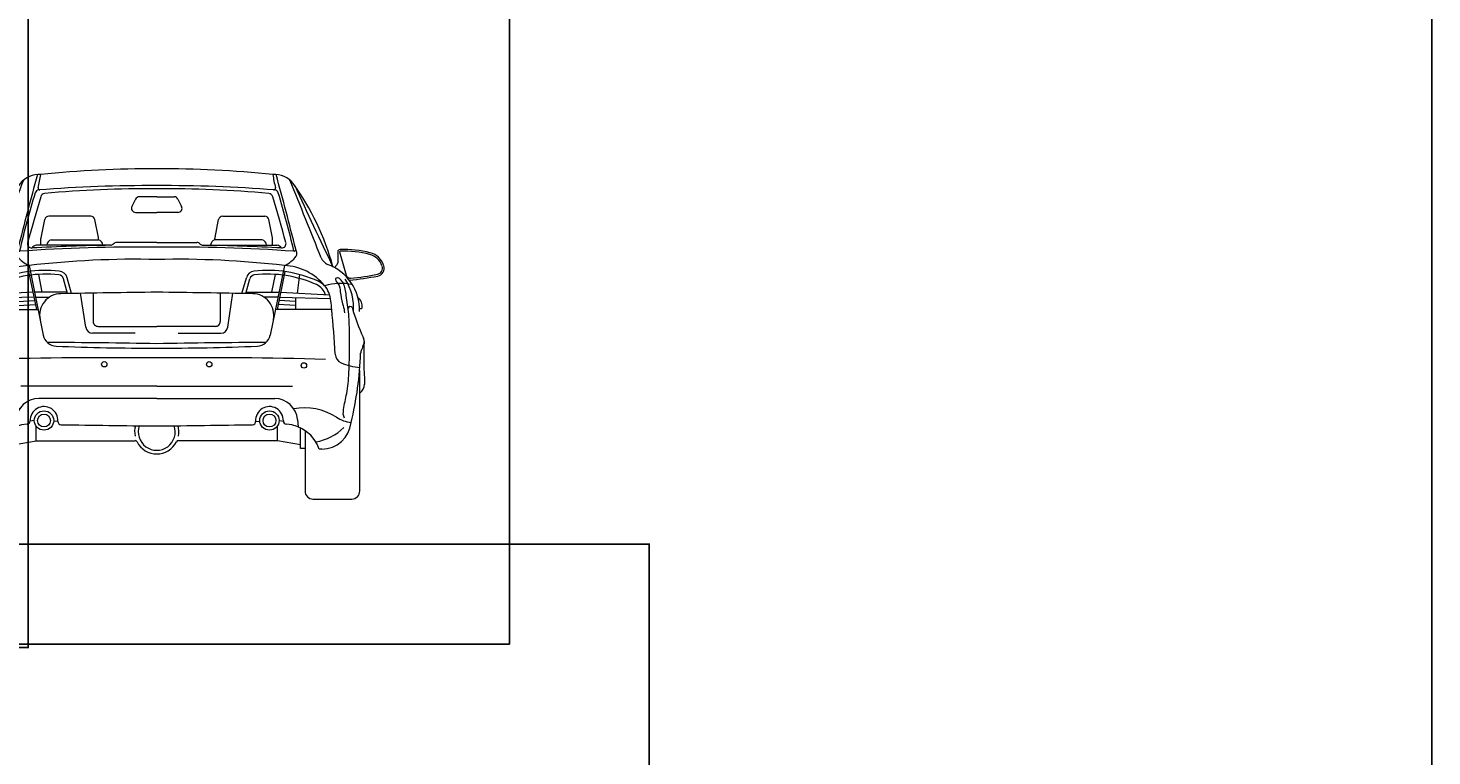
# Model space of a CAD drawing. Units: inches. Extents: x 1770 to 2988, y 1161 to 3221.
# Tile 37 of 44: x 2655 to 2988, y 2520 to 2693. Entities that reach past the tile are written whole.
import ezdxf

# ---------------------------------------------------------------- set-up
doc = ezdxf.new("R2010")
doc.units = ezdxf.units.IN
for name, color, linetype, lineweight in [('A-ANNO-DIMS', 2, 'Continuous', 18), ('A-ANNO-TTLB', 7, 'Continuous', 25), ('AUDI', 8, 'Continuous', 13)]:
    doc.layers.add(name, color=color, linetype=linetype, lineweight=lineweight)
doc.styles.get("Standard").update_dxf_attribs({"font": 'arial.ttf'})
doc.dimstyles.get("Standard").update_dxf_attribs({"dimtxt": 0.18, "dimasz": 0.18, "dimexe": 0.18, "dimexo": 0.0625, "dimgap": 0.09, "dimtad": 0, "dimtih": 1, "dimtoh": 1, "dimdec": 4, "dimzin": 0, "dimdsep": 46, "dimtxsty": 'Standard', "dimcen": 0.09, "dimadec": 0, "dimazin": 0, "dimtfac": 1, "dimtdec": 4, "dimtofl": 0, "dimtmove": 0, "dimatfit": 3, "dimfxl": 1, "dimtolj": 1, "dimtzin": 0, "dimarcsym": 0})

# ---------------------------------------------------------------- blocks, each defined once
blk = doc.blocks.new('CAR-SEDAN-REAR')
for p, q in [((48.82, 70.96), (47.96, 69.22)), ((53.84, 71.5), (49.7, 71.5)), ((53.84, 71.5), (57.98, 71.5)), ((58.85, 70.96), (59.72, 69.22)), ((38.23, 66.92), (28.28, 66.92)), ((48.83, 67.81), (53.84, 67.81)), ((58.85, 67.81), (53.84, 67.81)), ((69.45, 66.92), (79.4, 66.92)), ((26.45, 61.8), (27.32, 66.14)), ((40.05, 61.84), (39.18, 66.14)), ((67.63, 61.84), (68.49, 66.14)), ((81.23, 61.8), (80.35, 66.14)), ((42.86, 60.02), (25.37, 60.02)), ((26.43, 60.02), (26.43, 61.6)), ((28.84, 61.32), (40.07, 61.32)), ((40.07, 61.32), (40.07, 61.65)), ((53.84, 60.68), (44.34, 60.68)), ((53.84, 60.68), (63.33, 60.68)), ((64.82, 60.02), (82.31, 60.02)), ((67.61, 61.32), (67.61, 61.65)), ((78.83, 61.32), (67.61, 61.32)), ((81.25, 60.02), (81.25, 61.6)), ((10.57, 58.46), (8.97, 52.97)), ((10.98, 58.46), (10.98, 55.88)), ((96.69, 58.46), (96.69, 55.88)), ((97.11, 58.46), (98.7, 52.97)), ((11.13, 55.5), (11.78, 54.75)), ((23.5, 53.8), (25.35, 44.82)), ((23.6, 55.23), (26.98, 38.75)), ((84.07, 55.23), (80.69, 38.75)), ((84.17, 53.8), (82.33, 44.82)), ((96.55, 55.5), (95.89, 54.75)), ((20.01, 53.09), (20.57, 48.7)), ((25.81, 53.15), (26.67, 48.92)), ((32.74, 48.6), (31.77, 52.11)), ((33.66, 48.62), (32.63, 52.35)), ((74.01, 48.62), (75.05, 52.35)), ((74.93, 48.6), (75.91, 52.11)), ((81.86, 53.15), (81, 48.92)), ((87.67, 53.09), (87.11, 48.7)), ((24.75, 47.73), (12.7, 47.41)), ((24.51, 48.92), (12.93, 48.28)), ((21.03, 47.63), (21.03, 44.82)), ((21.03, 46.7), (24.91, 46.94)), ((32.66, 48.92), (24.9, 48.92)), ((25.14, 47.73), (28.4, 47.73)), ((37.02, 40.63), (35.79, 48.66)), ((38.8, 48.71), (38.8, 41.97)), ((68.87, 48.71), (68.87, 41.97)), ((70.66, 40.63), (71.88, 48.66)), ((75.02, 48.92), (82.78, 48.92)), ((82.53, 47.73), (79.28, 47.73)), ((86.65, 46.7), (82.76, 46.94)), ((82.93, 47.73), (94.98, 47.41)), ((83.17, 48.92), (94.75, 48.28)), ((86.65, 47.63), (86.65, 44.82)), ((12.42, 44.82), (25.74, 44.82)), ((21.03, 45.76), (25.1, 46.01)), ((95.26, 44.82), (81.94, 44.82)), ((86.65, 45.76), (82.57, 46.01)), ((39.94, 40.83), (53.84, 40.85)), ((67.73, 40.83), (53.84, 40.85)), ((48.76, 39.24), (38.64, 39.24)), ((58.92, 39.24), (69.03, 39.24)), ((5.76, 1.88), (5.76, 30.37)), ((101.91, 1.88), (101.91, 30.37)), ((53.84, 26.71), (21.69, 26.71)), ((53.84, 26.71), (85.99, 26.71)), ((53.84, 23.76), (25.9, 23.76)), ((53.84, 23.76), (81.77, 23.76)), ((19.82, 11.92), (19.82, 16.83)), ((20.53, 18.8), (20.39, 17.08)), ((24.86, 18.57), (23.85, 18.45)), ((25.28, 13.8), (25.28, 17.25)), ((30.45, 18.32), (29.43, 18.4)), ((77.23, 18.32), (78.24, 18.4)), ((82.39, 13.8), (82.39, 17.25)), ((82.81, 18.57), (83.83, 18.45)), ((87.15, 18.8), (87.29, 17.08)), ((87.86, 11.92), (87.86, 16.83)), ((18.74, 16.2), (18.74, 1.88)), ((19.82, 12.84), (25.28, 13.8)), ((25.28, 13.8), (48.72, 13.8)), ((82.39, 13.8), (58.95, 13.8)), ((87.86, 12.84), (82.39, 13.8)), ((88.94, 16.2), (88.94, 1.88)), ((14.78, 11.78), (15.36, 11.78)), ((18.74, 11.92), (19.82, 11.92)), ((88.94, 11.92), (87.86, 11.92)), ((92.9, 11.78), (92.32, 11.78)), ((16.86, 0), (7.64, 0)), ((90.82, 0), (100.03, 0))]:
    blk.add_line(p, q)
for centre, radius in [((19.01, 31.6), 0.639), ((41.42, 31.88), 0.639), ((66.26, 31.88), 0.639), ((88.66, 31.6), 0.639), ((27.15, 18.57), 2.29), ((27.15, 18.57), 1.52), ((80.52, 18.57), 2.29), ((80.52, 18.57), 1.52)]:
    blk.add_circle(centre, radius)
for centre, radius, start, end in [((643.9, -95.37), 641.82, 164.4425, 166.06975), ((25.95, 71.16), 5.63, 85.7838, 141.6623), ((-17.33, 84), 44.29, 346.4979, 350.6005), ((54.04, -199.85), 278, 90.0409, 95.713), ((53.64, -199.85), 278, 84.287, 89.9591), ((81.73, 71.16), 5.63, 38.3377, 94.2162), ((125, 84), 44.29, 189.3995, 193.5021), ((-536.22, -95.37), 641.82, 13.93025, 15.5575), ((70.58, 39.12), 60.56, 144.0802, 164.861), ((-1004.9, 545.01), 1128.96, 334.27309, 335.34979), ((2905.78, -1097.48), 3112.89, 157.86428, 158.22937), ((26.01, 72.12), 1, 94.5001, 163.0632), ((26.15, 73.56), 0.428, 166.4979, 274.4568), ((51.95, -257.52), 331.66, 89.6747, 94.5001), ((50.83, -174.43), 247.82, 89.305, 95.4501), ((55.72, -257.52), 331.66, 85.4999, 90.3253), ((56.84, -174.43), 247.82, 84.5499, 90.695), ((81.53, 73.56), 0.428, 265.5432, 13.5021), ((81.66, 72.12), 1, 16.9368, 85.4999), ((-2798.1, -1097.48), 3112.89, 21.77063, 22.13572), ((37.09, 39.12), 60.56, 15.139, 35.9198), ((1112.58, 545.01), 1128.96, 204.65021, 205.72691), ((223.34, 12.02), 207.28, 163.0632, 167.011), ((423.22, -48.19), 414.5, 163.2127, 164.7772), ((27.39, 71.22), 1.06, 95.4501, 163.2127), ((49.7, 70.53), 0.975, 90, 153.5465), ((57.98, 70.53), 0.975, 26.4535, 90), ((80.28, 71.22), 1.06, 16.7873, 84.5499), ((-315.55, -48.19), 414.5, 15.2228, 16.7873), ((-115.67, 12.02), 207.28, 12.989, 16.9368), ((28.28, 65.95), 0.975, 90, 168.5881), ((38.23, 65.95), 0.975, 11.4119, 90), ((48.83, 68.78), 0.975, 153.5465, 270), ((58.85, 68.78), 0.975, 270, 26.4535), ((69.45, 65.95), 0.975, 90, 168.5881), ((79.4, 65.95), 0.975, 11.4119, 90), ((24.23, 60.38), 1, 164.7772, 273.0474), ((50.52, -433.5), 493.59, 90.8895, 93.0474), ((25.37, 58.77), 1.25, 90.0461, 150.7436), ((27.4, 61.6), 0.975, 168.5881, 180), ((29.25, 59.93), 1.44, 106.4998, 173.9283), ((39.09, 61.65), 0.975, 0, 11.4119), ((39.66, 59.93), 1.44, 6.0717, 73.5002), ((42.84, 61.02), 1, 270.8895, 315.2014), ((44.44, 59.44), 1.25, 94.4926, 135.2014), ((63.23, 59.44), 1.25, 44.7986, 85.5074), ((64.83, 61.02), 1, 224.7986, 269.1105), ((57.15, -433.5), 493.59, 86.9526, 89.1105), ((68.02, 59.93), 1.44, 106.4998, 173.9283), ((68.58, 61.65), 0.975, 168.5881, 180), ((78.42, 59.93), 1.44, 6.0717, 73.5002), ((80.27, 61.6), 0.975, 0, 11.4119), ((82.3, 58.77), 1.25, 29.2564, 89.9539), ((83.45, 60.38), 1, 266.9526, 15.2228), ((4.4, 53.87), 4.51, 104.0957, 161.674), ((4.4, 53.87), 4.09, 104.0957, 161.674), ((9.83, 32.25), 26.8, 88.7503, 104.0957), ((9.83, 32.25), 26.39, 88.7503, 104.0957), ((10.4, 58.46), 0.164, 0, 88.7503), ((10.4, 58.46), 0.577, 0, 88.7503), ((11.85, 58.46), 3.37, 298.1193, 335.5163), ((22.75, 57.94), 2.12, 148.8459, 175.6295), ((21.64, 58.03), 1, 175.6295, 217.0304), ((26.45, 61.66), 7.02, 217.0304, 246.1166), ((21.37, 59.04), 0.428, 166.0697, 273.9966), ((49.05, -337.24), 396.82, 89.3093, 93.9966), ((49.07, -161.34), 218.06, 88.7475, 96.7073), ((58.62, -337.24), 396.82, 86.0034, 90.6907), ((58.6, -161.34), 218.06, 83.2927, 91.2525), ((81.23, 61.66), 7.02, 293.8834, 322.9696), ((86.31, 59.04), 0.428, 266.0034, 13.9303), ((84.92, 57.94), 2.12, 4.3705, 31.1541), ((86.04, 58.03), 1, 322.9696, 4.3705), ((95.83, 58.46), 3.37, 204.4837, 241.8807), ((97.27, 58.46), 0.577, 91.2497, 180), ((97.27, 58.46), 0.164, 91.2497, 180), ((97.84, 32.25), 26.8, 75.9043, 91.2497), ((97.84, 32.25), 26.39, 75.9043, 91.2497), ((103.27, 53.87), 4.09, 18.326, 75.9043), ((103.27, 53.87), 4.51, 18.326, 75.9043), ((1.89, 54.6), 1.89, 162.3817, 258.997), ((9.28, 52.25), 9.64, 161.674, 162.3817), ((1.89, 54.6), 1.47, 162.3817, 258.997), ((17.21, 44.75), 11.38, 109.397, 181.9623), ((11.56, 55.88), 0.577, 180, 221.428), ((24.16, 42.31), 12.94, 92.4534, 141.0622), ((27.62, 24.7), 29.39, 83.8593, 114.1135), ((27.62, 24.7), 28.5, 83.8593, 114.1135), ((30.54, 51.77), 2.17, 15.5227, 83.8593), ((77.14, 51.77), 2.17, 96.1407, 164.4773), ((80.05, 24.7), 29.39, 65.8865, 96.1407), ((80.05, 24.7), 28.5, 65.8865, 96.1407), ((83.52, 42.31), 12.94, 38.9378, 87.5466), ((90.46, 44.75), 11.38, 358.0377, 70.603), ((96.12, 55.88), 0.577, 318.572, 0), ((105.79, 54.6), 1.47, 281.003, 17.6183), ((105.79, 54.6), 1.89, 281.003, 17.6183), ((98.4, 52.25), 9.64, 17.6183, 18.326), ((15.01, 122.09), 70.64, 258.997, 264.5122), ((15.01, 122.09), 70.22, 258.997, 264.1692), ((19.49, 45.28), 12.27, 146.8264, 184.9502), ((10.28, 37.96), 13.05, 72.9961, 102.2038), ((7.98, 53.25), 1.03, 264.1692, 343.8085), ((17.54, 47.23), 4.71, 114.1135, 159.9948), ((17.54, 47.23), 3.82, 114.1135, 163.1664), ((30.54, 51.77), 1.28, 15.5227, 83.8593), ((77.14, 51.77), 1.28, 96.1407, 164.4773), ((90.13, 47.23), 3.82, 16.8336, 65.8865), ((90.13, 47.23), 4.71, 20.0052, 65.8865), ((97.4, 37.96), 13.05, 77.7962, 107.0039), ((88.18, 45.28), 12.27, 355.0498, 33.1736), ((99.7, 53.25), 1.03, 196.1915, 275.8308), ((92.67, 122.09), 70.64, 275.4878, 281.003), ((92.67, 122.09), 70.22, 275.8308, 281.003), ((7.72, 45.59), 2.53, 127.0648, 188.1795), ((23.92, 44.9), 11.5, 159.9948, 180.4078), ((31.2, 43.49), 5.08, 91.0763, 191.5926), ((88.42, -3002.35), 3051.46, 90.64943, 91.0763), ((19.25, -3002.35), 3051.46, 88.9237, 89.35057), ((76.47, 43.49), 5.08, 348.4074, 88.9237), ((83.75, 44.9), 11.5, 359.5922, 20.0052), ((99.95, 45.59), 2.53, 351.8205, 52.9352), ((-40.22, 59.31), 49.83, 335.0061, 343.6424), ((5.4, 45.26), 0.184, 188.1795, 265.5447), ((5.96, 52.47), 7.42, 265.5447, 269.0559), ((86.52, 37.3), 80.99, 174.9976, 178.3487), ((8.04, 45.01), 0.519, 13.0469, 148.7544), ((182.84, 26.36), 171.42, 173.8158, 177.3495), ((-75.17, 26.36), 171.42, 2.6505, 6.1842), ((99.64, 45.01), 0.519, 31.2456, 166.9531), ((147.89, 59.31), 49.83, 196.3576, 204.9939), ((101.71, 52.47), 7.42, 270.9441, 274.4553), ((102.28, 45.26), 0.184, 274.4553, 351.8205), ((38.64, 40.88), 1.64, 188.6953, 270), ((39.94, 41.97), 1.14, 180, 270.0801), ((67.73, 41.97), 1.14, 269.9199, 0), ((69.03, 40.88), 1.64, 270, 351.3047), ((-109.4, 33.61), 114.21, 356.7448, 1.8553), ((6.82, 37.38), 2.07, 155.0061, 181.8553), ((30.15, 39.4), 3.23, 191.5926, 267.5409), ((11.27, -2447.69), 2484.8, 89.01848, 89.61606), ((96.4, -2447.69), 2484.8, 90.38394, 90.98152), ((77.52, 39.4), 3.23, 272.4591, 348.4074), ((100.86, 37.38), 2.07, 358.1447, 24.9939), ((217.07, 33.61), 114.21, 178.1447, 183.2552), ((86.52, 37.3), 80.99, 181.9837, 193.7227), ((9.23, 34.39), 2.38, 293.9425, 357.3495), ((43.39, -1053.12), 1086.55, 89.44927, 91.55649), ((51.43, 534.93), 499.22, 267.5409, 270.276), ((56.24, 534.93), 499.22, 269.724, 272.4591), ((64.28, -1053.12), 1086.55, 88.44351, 90.55073), ((98.45, 34.39), 2.38, 182.6505, 246.0575), ((21.16, 37.3), 80.99, 346.2773, 358.0163), ((5.04, 43.83), 12.7, 273.2699, 293.9425), ((102.64, 43.83), 12.7, 246.0575, 266.7301), ((7.46, 27.34), 2.84, 184.2077, 233.2585), ((100.21, 27.34), 2.84, 306.7415, 355.7923), ((25.9, 18.37), 5.39, 90, 175.3467), ((81.77, 18.37), 5.39, 4.6533, 90), ((18.99, 7.02), 14.55, 80.3869, 121.8355), ((27.15, 18.57), 3.3, 356.4752, 181.7411), ((80.52, 18.57), 3.3, 358.2589, 183.5248), ((88.69, 7.02), 14.55, 58.1645, 99.6131), ((6.88, 26.02), 7.99, 276.9357, 303.7276), ((14.83, 18.8), 7.02, 185.7841, 269.5996), ((18.34, 25.97), 12.64, 225.7709, 260.141), ((23.69, 8.92), 8.81, 93.5063, 161.053), ((23.11, 18.45), 0.743, 273.5063, 1.7411), ((31.19, 18.32), 0.743, 176.4752, 269.02), ((74.78, 2566.5), 2549.29, 269.01996, 269.52932), ((53.84, 15.9), 5.24, 164.039, 190.9633), ((53.84, 15.9), 4.37, 160.8842, 19.1158), ((32.9, 2566.5), 2549.29, 270.47068, 270.98004), ((53.84, 15.9), 5.24, 349.0367, 15.961), ((76.49, 18.32), 0.743, 270.98, 3.5248), ((84.57, 18.45), 0.743, 178.2589, 266.4937), ((83.98, 8.92), 8.81, 18.947, 86.4937), ((89.33, 25.97), 12.64, 279.859, 314.2291), ((92.85, 18.8), 7.02, 270.4004, 354.2159), ((100.8, 26.02), 7.99, 236.2724, 263.0643), ((48.72, 13.3), 0.504, 26.9755, 90), ((53.84, 15.9), 5.24, 206.9755, 333.0245), ((58.95, 13.3), 0.504, 90, 153.0245), ((7.64, 1.88), 1.88, 180, 270), ((16.86, 1.88), 1.88, 270, 0), ((90.82, 1.88), 1.88, 180, 270), ((100.03, 1.88), 1.88, 270, 0)]:
    blk.add_arc(centre, radius, start, end)
for points, knots in [([(9.37, 19.11), (9.75, 19.68), (9.62, 21.86), (8.68, 25.22), (8.18, 31.21), (8.19, 37.44), (8.27, 43.61), (8.91, 47.62), (9.28, 50.6), (10.23, 51.92), (10.94, 52.45), (11.91, 52.04), (10.48, 50.68), (10.42, 48.79), (10.02, 46.51), (9.45, 44.93), (9.41, 44.2), (9.41, 44.07)], [0, 0, 0, 0, 2.067985, 5.917661, 10.817048, 19.839487, 24.72726, 29.230389, 32.162056, 33.39317, 34.11598, 34.608356, 35.870676, 37.977272, 40.803487, 42.600574, 42.988867, 42.988867, 42.988867, 42.988867]), ([(98.31, 19.11), (97.92, 19.68), (98.06, 21.86), (98.99, 25.22), (99.49, 31.21), (99.48, 37.44), (99.4, 43.61), (98.77, 47.62), (98.4, 50.6), (97.44, 51.92), (96.74, 52.45), (95.77, 52.04), (97.19, 50.68), (97.26, 48.79), (97.66, 46.51), (98.22, 44.93), (98.26, 44.2), (98.26, 44.07)], [0, 0, 0, 0, 2.067985, 5.917661, 10.817048, 19.839487, 24.72726, 29.230389, 32.162056, 33.39317, 34.11598, 34.608356, 35.870676, 37.977272, 40.803487, 42.600574, 42.988867, 42.988867, 42.988867, 42.988867]), ([(4.75, 37.31), (4.75, 37.31), (4.77, 36.84), (5.1, 36.19), (5.34, 35.23), (5.58, 34.73), (5.58, 34.43)], [0, 0, 0, 0, 0.000002, 1.419502, 2.081106, 3.002245, 3.002245, 3.002245, 3.002245]), ([(102.92, 37.31), (102.92, 37.31), (102.9, 36.84), (102.57, 36.19), (102.33, 35.23), (102.09, 34.73), (102.09, 34.43)], [0, 0, 0, 0, 0.000002, 1.419502, 2.081106, 3.002245, 3.002245, 3.002245, 3.002245])]:
    blk.add_open_spline(points, degree=3, knots=knots)
blk = doc.blocks.new('*D56')
at = {"layer": 'A-ANNO-DIMS', "color": 0, "lineweight": -2, "transparency": 16777216}
for p, q in [((1971.53, 2506.34), (1971.53, 2570.7)), ((1971.71, 2570.52), (2386.59, 2570.52)), ((2802.26, 2570.52), (2387.38, 2570.52)), ((2802.44, 2506.34), (2802.44, 2570.7))]:
    blk.add_line(p, q, dxfattribs=at)
at = {"layer": 'A-ANNO-DIMS', "color": 0, "transparency": 16777216}
for points in [[(1971.71, 2570.55), (1971.71, 2570.49), (1971.53, 2570.52)], [(2802.26, 2570.55), (2802.26, 2570.49), (2802.44, 2570.52)]]:
    blk.add_solid(points, dxfattribs=at)
at = {"layer": 'Defpoints', "color": 0, "transparency": 16777216}
for p in [(2802.44, 2570.52), (1971.53, 2506.27), (2802.44, 2506.27)]:
    blk.add_point(p, dxfattribs=at)
at = {"layer": 'A-ANNO-DIMS', "color": 0, "transparency": 16777216, "insert": (2386.99, 2570.52), "char_height": 0.18, "attachment_point": 5}
blk.add_mtext('\\A1;830.9', dxfattribs=at)
blk = doc.blocks.new('*D93')
at = {"layer": 'A-ANNO-DIMS', "color": 0, "lineweight": -2, "transparency": 16777216}
for p, q in [((2181.44, 2704.23), (2181.44, 2545.88)), ((2655.44, 2704.23), (2655.44, 2545.88)), ((2181.62, 2546.06), (2418.15, 2546.06)), ((2655.26, 2546.06), (2418.74, 2546.06))]:
    blk.add_line(p, q, dxfattribs=at)
at = {"layer": 'A-ANNO-DIMS', "color": 0, "transparency": 16777216}
for points in [[(2181.62, 2546.09), (2181.62, 2546.03), (2181.44, 2546.06)], [(2655.26, 2546.09), (2655.26, 2546.03), (2655.44, 2546.06)]]:
    blk.add_solid(points, dxfattribs=at)
at = {"layer": 'Defpoints', "color": 0, "transparency": 16777216}
for p in [(2181.44, 2704.3), (2655.44, 2704.3), (2655.44, 2546.06)]:
    blk.add_point(p, dxfattribs=at)
at = {"layer": 'A-ANNO-DIMS', "color": 0, "transparency": 16777216, "insert": (2418.44, 2546.06), "char_height": 0.18, "attachment_point": 5}
blk.add_mtext('\\A1;474', dxfattribs=at)

msp = doc.modelspace()

# ---------------------------------------------------------------- linework, layer by layer
at = {"layer": 'A-ANNO-TTLB'}
for points in [[(1769.9155, 3221.2788), (2987.7567, 3221.2788), (2987.7567, 1161.1516), (1769.9155, 1161.1516)], [(2073.6202, 3129.9468), (2769.3644, 3129.9468), (2769.3644, 2546.8952), (2073.6202, 2546.8952)]]:
    msp.add_lwpolyline(points, close=True, dxfattribs=at)

# ---------------------------------------------------------------- block references
at = {"layer": 'AUDI'}
msp.add_blockref('CAR-SEDAN-REAR', (2632.0624, 2581.1972), dxfattribs=at)

# ---------------------------------------------------------------- dimensions: what is measured, and where the dimension line sits
at = {"layer": 'A-ANNO-DIMS'}
for base, p1, p2, override, picture, middle in [((2655.443, 2546.0579), (2181.443, 2704.2969), (2655.443, 2704.2969), {"dimdec": 0, "dimlfac": 1, "dimrnd": 0, "dimzin": 0, "dimdsep": 46, "dimlunit": 2}, '*D93', (2418.443, 2546.0579)), ((2802.4374, 2570.5247), (1971.5344, 2506.2747), (2802.4374, 2506.2747), {"dimdec": 1, "dimlfac": 1, "dimrnd": 0, "dimzin": 0, "dimdsep": 46, "dimlunit": 2}, '*D56', (2386.9859, 2570.5247))]:
    dim = msp.add_linear_dim(base=base, p1=p1, p2=p2, dimstyle='Standard', override=override, dxfattribs=at)
    dim.commit()
    dim.dimension.update_dxf_attribs({"geometry": picture, "text_midpoint": middle})

doc.saveas('drawing.dxf')
